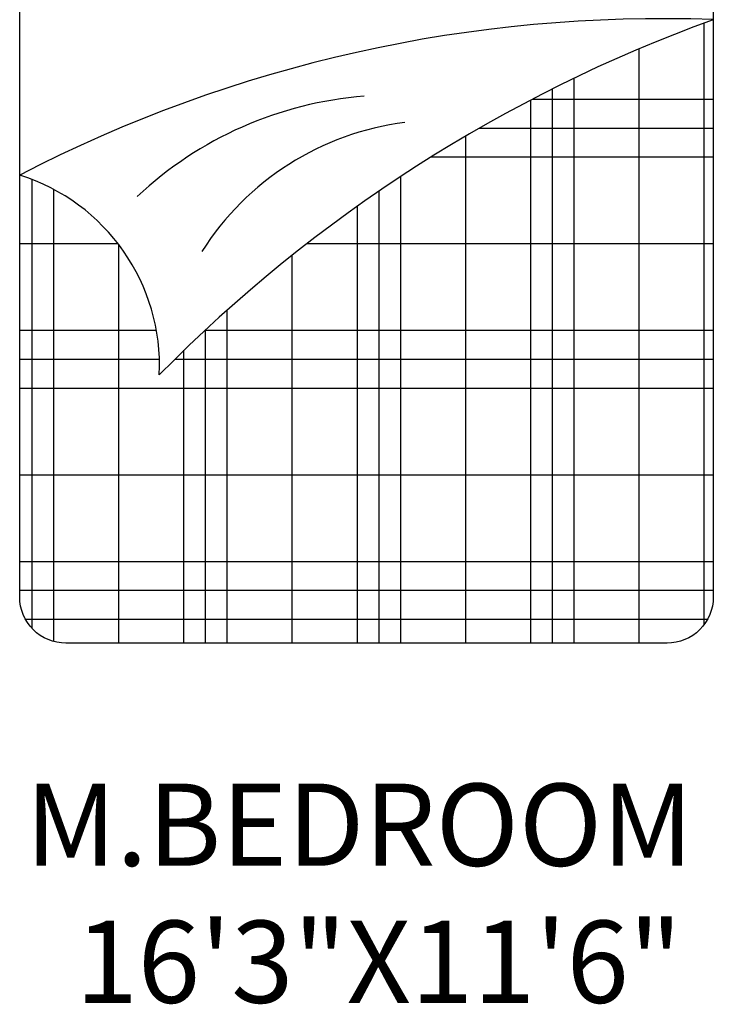
# Model space of a CAD drawing. Units: inches. Extents: x 3064 to 19385, y 846 to 15425.
# Tile 88 of 108: x 7309 to 7368, y 1289 to 1373. Entities that reach past the tile are written whole.
import ezdxf

# ---------------------------------------------------------------- set-up
doc = ezdxf.new("R2010")
doc.units = ezdxf.units.IN
doc.layers.add('A-AREA-IDEN', color=3, linetype='Continuous', lineweight=18)
doc.layers.add('A-FLOR-FIXT', color=9, linetype='Continuous', lineweight=18)
doc.layers.add('BLOCK', color=6, linetype='Continuous')
doc.styles.get("Standard").update_dxf_attribs({"font": 'arial.ttf'})

# ---------------------------------------------------------------- blocks, each defined once
blk = doc.blocks.new('*X5')
at = {"color": 0}
for p, q in [((276.598, 451.25), (280.51, 451.25)), ((275.455, 450.625), (280.51, 450.625)), ((274.411, 450), (280.51, 450)), ((265.51, 448.125), (267.634, 448.125)), ((271.723, 448.125), (280.51, 448.125)), ((265.51, 446.25), (268.465, 446.25)), ((269.519, 446.25), (280.51, 446.25)), ((265.51, 445.625), (268.531, 445.625)), ((268.866, 445.625), (280.51, 445.625)), ((265.51, 445), (280.51, 445)), ((265.51, 443.125), (280.51, 443.125)), ((265.51, 441.25), (280.51, 441.25)), ((265.51, 440.625), (280.51, 440.625)), ((265.634, 440), (280.386, 440))]:
    blk.add_line(p, q, dxfattribs=at)
blk = doc.blocks.new('*X6')
at = {"color": 0}
for p, q in [((280.312, 439.886), (280.312, 452.896)), ((278.906, 439.482), (278.906, 452.338)), ((277.5, 439.482), (277.5, 451.702)), ((277.031, 439.482), (277.031, 451.471)), ((276.562, 439.482), (276.562, 451.231)), ((275.156, 439.482), (275.156, 450.451)), ((265.781, 439.797), (265.781, 449.511)), ((273.75, 439.482), (273.75, 449.576)), ((266.25, 439.517), (266.25, 449.296)), ((273.281, 439.482), (273.281, 449.261)), ((272.812, 439.482), (272.812, 448.934)), ((267.656, 439.482), (267.656, 448.095)), ((271.406, 439.482), (271.406, 447.876)), ((270, 439.482), (270, 446.689)), ((269.531, 439.482), (269.531, 446.262)), ((269.062, 439.482), (269.062, 445.817))]:
    blk.add_line(p, q, dxfattribs=at)
blk = doc.blocks.new('A$C52E67D0D')
at = {"layer": 'BLOCK'}
blk.add_lwpolyline([(1901, 0), (601, 0, -0.414214), (501, 100), (501, 1700, -0.414214), (601, 1800), (1901, 1800, -0.414214), (2001, 1700), (2001, 100, -0.414214)], format="xyb", close=True, dxfattribs=at)
for centre, radius, start, end in [((1888.6, -1664.5), 3015.3, 87.8642, 117.4001), ((3101, -1685.8), 3227.7, 109.926, 135.3977), ((1308.8, 377.9), 807.6, 94.4436, 133.2788), ((1410.8, 520.2), 610.8, 97.2157, 147.6656), ((371.4, 600.4), 432, 357.3792, 72.5379)]:
    blk.add_arc(centre, radius, start, end, dxfattribs=at)
at = {"layer": 'BLOCK', "xscale": 100, "yscale": 100, "zscale": 100}
for name in ['*X6', '*X5']:
    blk.add_blockref(name, (-26050, -43948.2), dxfattribs=at)

msp = doc.modelspace()

# ---------------------------------------------------------------- block references
at = {"layer": 'A-FLOR-FIXT', "xscale": 0.039370099999992, "yscale": 0.039370099999992, "zscale": 0.039370099999992}
msp.add_blockref('A$C52E67D0D', (7288.953, 1319.474), dxfattribs=at)

# ---------------------------------------------------------------- texts
at = {"layer": 'A-AREA-IDEN', "insert": (7309.154, 1307.513), "char_height": 7, "attachment_point": 1}
msp.add_mtext_dynamic_manual_height_columns('M.BEDROOM\\P  16\'3"X11\'6"', width=67.59241, gutter_width=12.5, heights=[0], dxfattribs=at)

doc.saveas('drawing.dxf')
